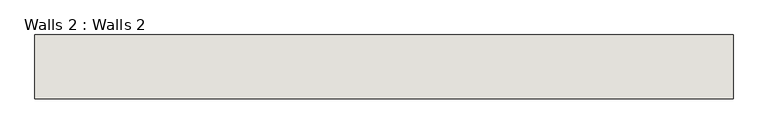
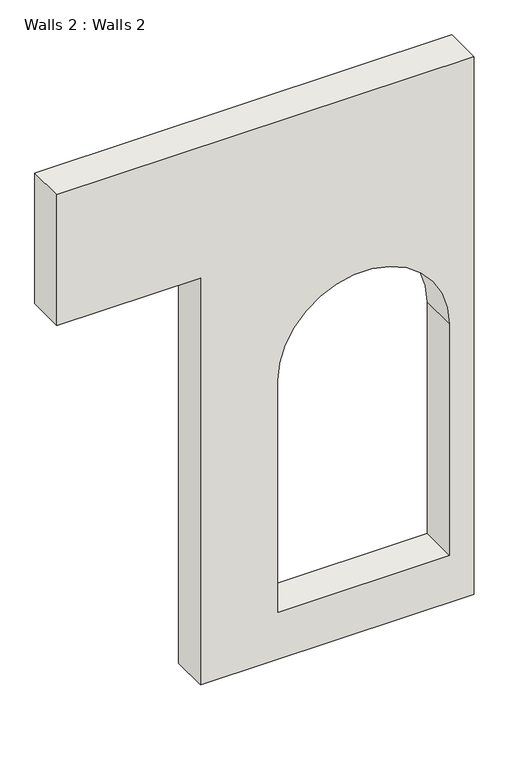
"""IFC4 building model written with IfcOpenShell, lengths in millimetres: wall geometry, Walls 2 : Walls 2."""

from ifc_helpers import new_model, si_unit, point, frame, frame_2d, origin, place, context, project, spatial, polyline, circle_curve, trimmed, segment, composite_curve, outline, extrude, source, transform, mapped, element, save


def walls_2_walls_2_f3eab2de(model_context):
    return source(origin(), model_context, "Body", "SweptSolid", [
        extrude(outline(polyline([(6096.0, -429.4748459), (6096.0, 721.7647473), (2648.0, 721.7647473), (2648.0, 2911.6217382), (7202.5236053, 2911.6217382), (7202.5236053, -429.4748459), (6096.0, -429.4748459)]), holes=[composite_curve([segment(polyline([(3048.0, 1342.1247411), (5010.2, 1342.1247411)]), True, "CONTINUOUS"), segment(trimmed(circle_curve(frame_2d((5010.2, 2027.9247411)), 685.8), [point((5010.2, 1342.1247411))], [point((5010.2, 2713.7247411))], True, "CARTESIAN"), True, "CONTINUOUS"), segment(polyline([(5010.2, 2713.7247411), (3048.0, 2713.7247411), (3048.0, 1342.1247411)]), True, "CONTINUOUS")], self_intersect=False)]), frame((0.0, -893.9851555, 0.0), z_axis=(0.0, 1.0, 0.0), x_axis=(0.0, 0.0, 1.0)), (0.0, 0.0, 1.0), 304.8),
    ])


if __name__ == "__main__":
    model = new_model("IFC4")
    model_context = context("Model", 3, world=origin())
    ifc_project = project(units=[si_unit("LENGTHUNIT", "METRE", prefix="MILLI")], contexts=[model_context])
    site = spatial("IfcSite", under=ifc_project)
    building = spatial("IfcBuilding", under=site)
    placement = place(None, origin())
    walls_2_walls_2_shape = walls_2_walls_2_f3eab2de(model_context)
    element("IfcWall", 1, ObjectType="Walls 2 : Walls 2", at=placement, inside=building, context=model_context, shape_type="MappedRepresentation", body=[
        mapped(walls_2_walls_2_shape, transform((0.0, 0.0, 0.0), x_axis=(1.0, 0.0, 0.0), y_axis=(0.0, 1.0, 0.0), z_axis=(0.0, 0.0, 1.0))),
    ])
    save(model, "model.ifc")

# Revit data of these elements
# Element 1 (IfcWall, "Walls 2 : Walls 2")
#   Materials on its faces: "Default Wall"
# Materials
#   "Default Wall": colour RGB 80 80 80, transparency 0
